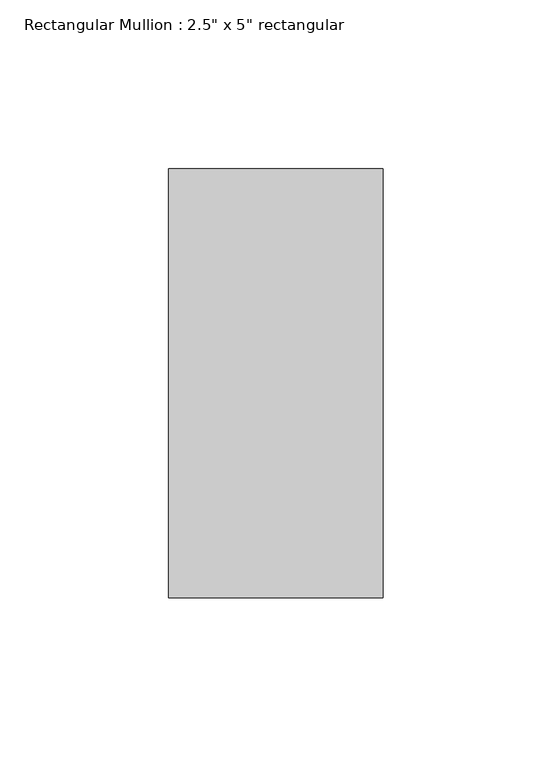
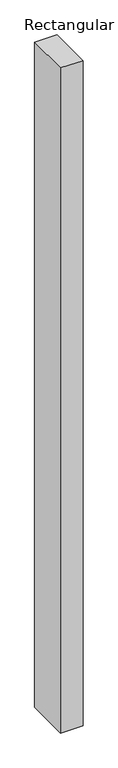
"""IFC4 building model written with IfcOpenShell, lengths in millimetres: member geometry."""

from ifc_helpers import new_model, si_unit, frame, origin, place, context, project, spatial, polyline, outline, extrude, source, transform, mapped, element, save


def member_2d710983(model_context):
    return source(origin(), model_context, "Body", "SweptSolid", [
        extrude(outline(polyline([(31.75, 63.5), (31.75, -63.5), (-31.75, -63.5), (-31.75, 63.5), (31.75, 63.5)])), frame((0.0, 0.0, -1995.867321), z_axis=(0.0, 0.0, 1.0), x_axis=(1.0, 0.0, 0.0)), (0.0, 0.0, 1.0), 1995.867321),
    ])


if __name__ == "__main__":
    model = new_model("IFC4")
    model_context = context("Model", 3, world=origin())
    ifc_project = project(units=[si_unit("LENGTHUNIT", "METRE", prefix="MILLI")], contexts=[model_context])
    site = spatial("IfcSite", under=ifc_project)
    building = spatial("IfcBuilding", under=site)
    placement = place(None, origin())
    member_shape = member_2d710983(model_context)
    element("IfcMember", 1, ObjectType="Rectangular Mullion : 2.5\" x 5\" rectangular", at=placement, inside=building, context=model_context, shape_type="MappedRepresentation", body=[
        mapped(member_shape, transform((0.0, 0.0, 0.0), x_axis=(1.0, 0.0, 0.0), y_axis=(0.0, 1.0, 0.0), z_axis=(0.0, 0.0, 1.0))),
    ])
    save(model, "model.ifc")

# Revit data of these elements
# Type "Rectangular Mullion : 2.5\" x 5\" rectangular"
#   built-in parameter 1007304 = 0.416667 (stored number, unit not read)
#   built-in parameter 1007301 = 0.104167 (stored number, unit not read)
#   built-in parameter 1007300 = 0.104167 (stored number, unit not read)
# Element 1 (IfcMember, "Rectangular Mullion : 2.5\" x 5\" rectangular")
#   Materials on its faces: "Aluminum"
# Materials
#   "Aluminum": class "Metal", colour RGB 247 247 247, transparency 0, Description = "Aluminum 6061", Cost = 0
